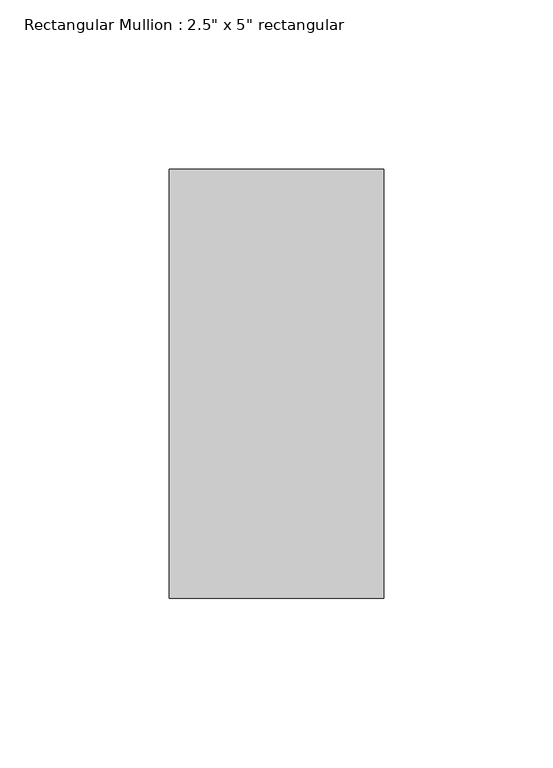
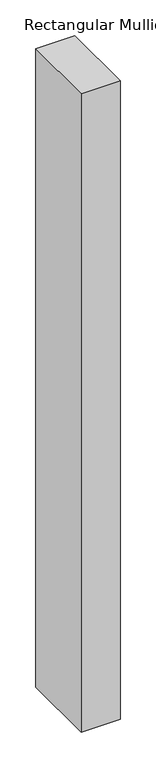
"""IFC4 building model written with IfcOpenShell, lengths in millimetres: member geometry."""

from ifc_helpers import new_model, si_unit, frame, origin, place, context, project, spatial, polyline, outline, extrude, source, transform, mapped, element, save


def member_867fe1e1(model_context):
    return source(origin(), model_context, "Body", "SweptSolid", [
        extrude(outline(polyline([(31.75, 63.5), (31.75, -63.5), (-31.75, -63.5), (-31.75, 63.5), (31.75, 63.5)])), frame((0.0, 0.0, -1092.2), z_axis=(0.0, 0.0, 1.0), x_axis=(1.0, 0.0, 0.0)), (0.0, 0.0, 1.0), 1092.2),
    ])


if __name__ == "__main__":
    model = new_model("IFC4")
    model_context = context("Model", 3, world=origin())
    ifc_project = project(units=[si_unit("LENGTHUNIT", "METRE", prefix="MILLI")], contexts=[model_context])
    site = spatial("IfcSite", under=ifc_project)
    building = spatial("IfcBuilding", under=site)
    placement = place(None, origin())
    member_shape = member_867fe1e1(model_context)
    element("IfcMember", 1, ObjectType="Rectangular Mullion : 2.5\" x 5\" rectangular", at=placement, inside=building, context=model_context, shape_type="MappedRepresentation", body=[
        mapped(member_shape, transform((0.0, 0.0, 0.0), x_axis=(1.0, 0.0, 0.0), y_axis=(0.0, 1.0, 0.0), z_axis=(0.0, 0.0, 1.0))),
    ])
    save(model, "model.ifc")

# Revit data of these elements
# Type "Rectangular Mullion : 2.5\" x 5\" rectangular"
#   built-in parameter 1007304 = 0.416667 (stored number, unit not read)
#   built-in parameter 1007301 = 0.104167 (stored number, unit not read)
#   built-in parameter 1007300 = 0.104167 (stored number, unit not read)
# Element 1 (IfcMember, "Rectangular Mullion : 2.5\" x 5\" rectangular")
#   Materials on its faces: "Aluminum"
# Materials
#   "Aluminum": class "Metal", colour RGB 247 247 247, transparency 0, Description = "Aluminum 6061", Cost = 0
